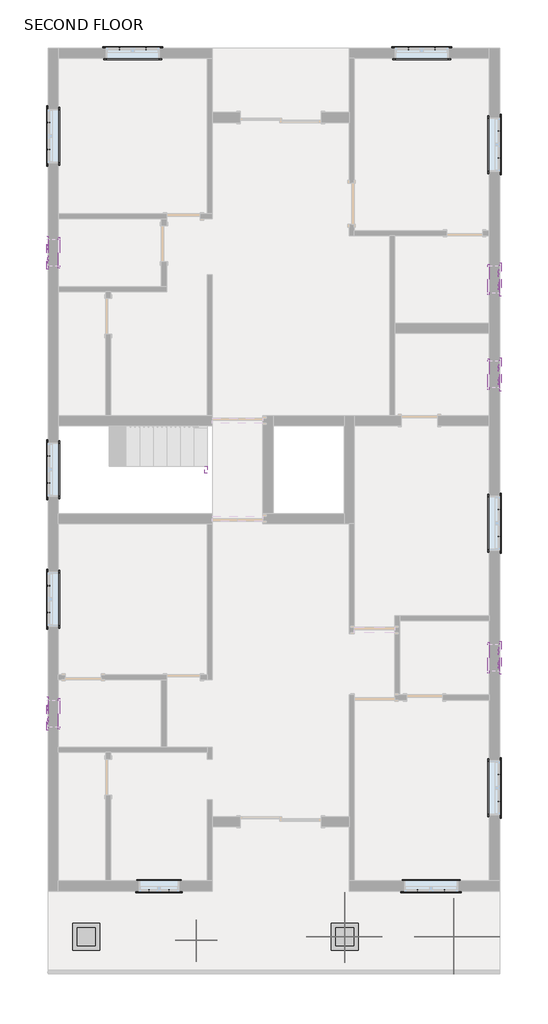
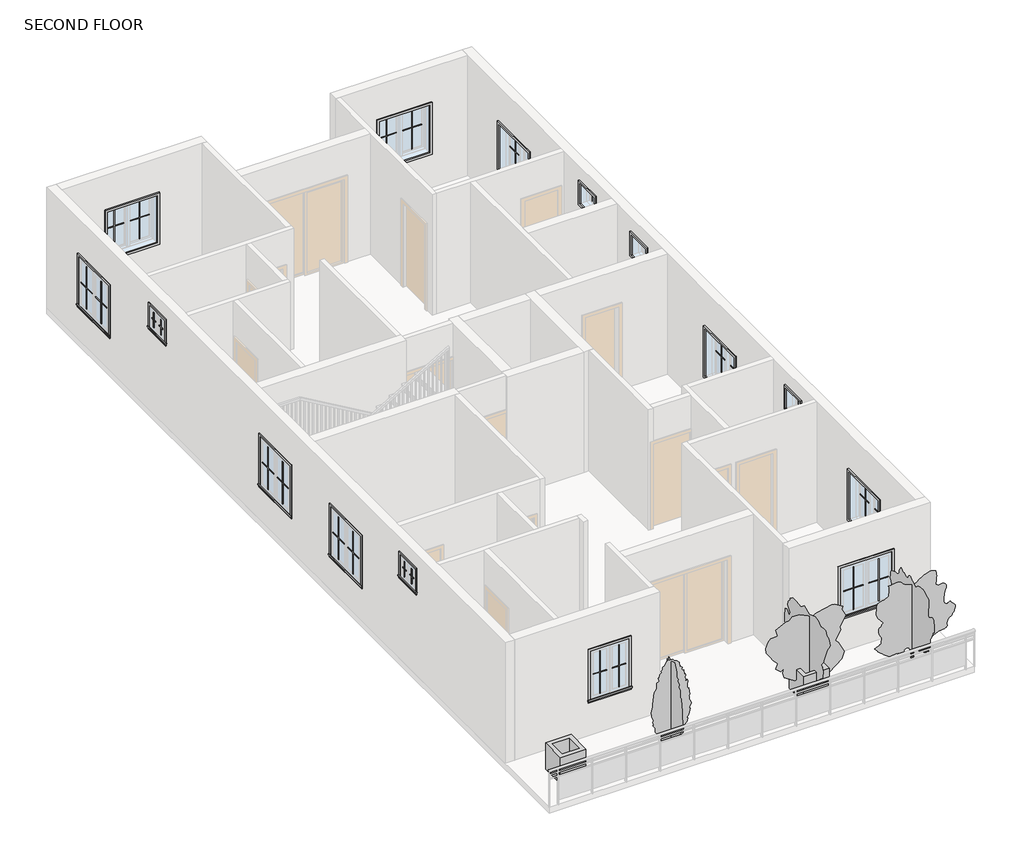
# One storey, part 4 of 4: 60 proxies, 5 geographic elements, 1 railing.
"""IFC4 building model written with IfcOpenShell, lengths in millimetres."""

from ifc_helpers import new_model, si_unit, frame, origin, place, context, project, spatial, polyline, outline, extrude, transform, mapped, element, save
from components import muntin_pattern_2x2_muntin_pattern_2x2_4dfeb3f3, muntin_pattern_2x2_muntin_pattern_2x2_e852a7e4, muntin_pattern_2x2_muntin_pattern_2x2_1acec82f, muntin_pattern_2x2_muntin_pattern_2x2_43d02eee, muntin_pattern_2x2_muntin_pattern_2x2_653c8599, muntin_pattern_2x2_muntin_pattern_2x2_c179cf80, trim_window_exterior_flat_with_sill_7cfdd449, trim_window_exterior_flat_with_sill_e4b28ec3, trim_window_exterior_flat_with_sill_e6f34eb5, trim_window_interior_flat_picture_frame_f1e0b15b, trim_window_interior_flat_picture_frame_39ff4276, trim_window_interior_flat_picture_frame_9a74d23d, planter_2_x2_5b049b04, rpc_tree_conifer_chinese_juniper_7_2_1b9786cd, rpc_tree_fall_american_beech_20_7ed35302, rpc_tree_fall_service_berry_25_c2e4521a

model = new_model("IFC4")

# Units and contexts
model_context = context("Model", 3, world=origin())
ifc_project = project(units=[si_unit("LENGTHUNIT", "METRE", prefix="MILLI")], contexts=[model_context])

# Site, building, storey
site = spatial("IfcSite", under=ifc_project)
building = spatial("IfcBuilding", under=site)
storey = spatial("IfcBuildingStorey", under=building, Name="SECOND FLOOR", Elevation=6400.8)

# Proxies
placement = place(None, origin())
muntin_pattern_2x2_muntin_pattern_2x2_shape = muntin_pattern_2x2_muntin_pattern_2x2_4dfeb3f3(model_context)
element("IfcBuildingElementProxy", 1, Name="Muntin Pattern_2x2 : Muntin Pattern_2x2", ObjectType="Muntin Pattern_2x2 : Muntin Pattern_2x2", at=placement, inside=storey, context=model_context, shape_type="MappedRepresentation", body=[
    mapped(muntin_pattern_2x2_muntin_pattern_2x2_shape, transform((-4756.4414041, 10049.2903263, 7385.05), x_axis=(1.0, 0.0, 0.0), y_axis=(0.0, 1.0, 0.0), z_axis=(0.0, 0.0, 1.0))),
])
element("IfcBuildingElementProxy", 2, Name="Muntin Pattern_2x2 : Muntin Pattern_2x2", ObjectType="Muntin Pattern_2x2 : Muntin Pattern_2x2", at=placement, inside=storey, context=model_context, shape_type="MappedRepresentation", body=[
    mapped(muntin_pattern_2x2_muntin_pattern_2x2_shape, transform((-6348.7039041, 7774.4028263, 7385.05), x_axis=(0.0, 1.0, 0.0), y_axis=(-1.0, 0.0, 0.0), z_axis=(0.0, 0.0, 1.0))),
])
element("IfcBuildingElementProxy", 3, Name="Muntin Pattern_2x2 : Muntin Pattern_2x2", ObjectType="Muntin Pattern_2x2 : Muntin Pattern_2x2", at=placement, inside=storey, context=model_context, shape_type="MappedRepresentation", body=[
    mapped(muntin_pattern_2x2_muntin_pattern_2x2_shape, transform((-6348.7039041, -2664.9971737, 7385.05), x_axis=(0.0, 1.0, 0.0), y_axis=(-1.0, 0.0, 0.0), z_axis=(0.0, 0.0, 1.0))),
])
element("IfcBuildingElementProxy", 4, Name="Muntin Pattern_2x2 : Muntin Pattern_2x2", ObjectType="Muntin Pattern_2x2 : Muntin Pattern_2x2", at=placement, inside=storey, context=model_context, shape_type="MappedRepresentation", body=[
    mapped(muntin_pattern_2x2_muntin_pattern_2x2_shape, transform((2575.0232801, -8930.8596737, 7385.05), x_axis=(-1.0, 0.0, 0.0), y_axis=(0.0, -1.0, 0.0), z_axis=(0.0, 0.0, 1.0))),
])
element("IfcBuildingElementProxy", 5, Name="Muntin Pattern_2x2 : Muntin Pattern_2x2", ObjectType="Muntin Pattern_2x2 : Muntin Pattern_2x2", at=placement, inside=storey, context=model_context, shape_type="MappedRepresentation", body=[
    mapped(muntin_pattern_2x2_muntin_pattern_2x2_shape, transform((3804.9460959, -6313.0721737, 7385.05), x_axis=(0.0, -1.0, 0.0), y_axis=(1.0, 0.0, 0.0), z_axis=(0.0, 0.0, 1.0))),
])
element("IfcBuildingElementProxy", 6, Name="Muntin Pattern_2x2 : Muntin Pattern_2x2", ObjectType="Muntin Pattern_2x2 : Muntin Pattern_2x2", at=placement, inside=storey, context=model_context, shape_type="MappedRepresentation", body=[
    mapped(muntin_pattern_2x2_muntin_pattern_2x2_shape, transform((3804.9460959, -344.0721737, 7385.05), x_axis=(0.0, -1.0, 0.0), y_axis=(1.0, 0.0, 0.0), z_axis=(0.0, 0.0, 1.0))),
])
element("IfcBuildingElementProxy", 7, Name="Muntin Pattern_2x2 : Muntin Pattern_2x2", ObjectType="Muntin Pattern_2x2 : Muntin Pattern_2x2", at=placement, inside=storey, context=model_context, shape_type="MappedRepresentation", body=[
    mapped(muntin_pattern_2x2_muntin_pattern_2x2_shape, transform((3804.9460959, 8190.3278263, 7385.05), x_axis=(0.0, -1.0, 0.0), y_axis=(1.0, 0.0, 0.0), z_axis=(0.0, 0.0, 1.0))),
])
element("IfcBuildingElementProxy", 8, Name="Muntin Pattern_2x2 : Muntin Pattern_2x2", ObjectType="Muntin Pattern_2x2 : Muntin Pattern_2x2", at=placement, inside=storey, context=model_context, shape_type="MappedRepresentation", body=[
    mapped(muntin_pattern_2x2_muntin_pattern_2x2_shape, transform((1758.6585959, 10049.2903263, 7385.05), x_axis=(1.0, 0.0, 0.0), y_axis=(0.0, 1.0, 0.0), z_axis=(0.0, 0.0, 1.0))),
])
element("IfcBuildingElementProxy", 9, Name="Muntin Pattern_2x2 : Muntin Pattern_2x2", ObjectType="Muntin Pattern_2x2 : Muntin Pattern_2x2", at=placement, inside=storey, context=model_context, shape_type="MappedRepresentation", body=[
    mapped(muntin_pattern_2x2_muntin_pattern_2x2_shape, transform((-6348.7039041, 256.0028263, 7385.05), x_axis=(0.0, 1.0, 0.0), y_axis=(-1.0, 0.0, 0.0), z_axis=(0.0, 0.0, 1.0))),
])
muntin_pattern_2x2_muntin_pattern_2x2_2_shape = muntin_pattern_2x2_muntin_pattern_2x2_e852a7e4(model_context)
element("IfcBuildingElementProxy", 10, Name="Muntin Pattern_2x2 : Muntin Pattern_2x2", ObjectType="Muntin Pattern_2x2 : Muntin Pattern_2x2", at=placement, inside=storey, context=model_context, shape_type="MappedRepresentation", body=[
    mapped(muntin_pattern_2x2_muntin_pattern_2x2_2_shape, transform((-4150.0164041, 10049.2903263, 7385.05), x_axis=(-1.0, 0.0, 0.0), y_axis=(0.0, -1.0, 0.0), z_axis=(0.0, 0.0, 1.0))),
])
element("IfcBuildingElementProxy", 11, Name="Muntin Pattern_2x2 : Muntin Pattern_2x2", ObjectType="Muntin Pattern_2x2 : Muntin Pattern_2x2", at=placement, inside=storey, context=model_context, shape_type="MappedRepresentation", body=[
    mapped(muntin_pattern_2x2_muntin_pattern_2x2_2_shape, transform((-6348.7039041, 8380.8278263, 7385.05), x_axis=(0.0, -1.0, 0.0), y_axis=(1.0, 0.0, 0.0), z_axis=(0.0, 0.0, 1.0))),
])
element("IfcBuildingElementProxy", 12, Name="Muntin Pattern_2x2 : Muntin Pattern_2x2", ObjectType="Muntin Pattern_2x2 : Muntin Pattern_2x2", at=placement, inside=storey, context=model_context, shape_type="MappedRepresentation", body=[
    mapped(muntin_pattern_2x2_muntin_pattern_2x2_2_shape, transform((-6348.7039041, -2058.5721737, 7385.05), x_axis=(0.0, -1.0, 0.0), y_axis=(1.0, 0.0, 0.0), z_axis=(0.0, 0.0, 1.0))),
])
element("IfcBuildingElementProxy", 13, Name="Muntin Pattern_2x2 : Muntin Pattern_2x2", ObjectType="Muntin Pattern_2x2 : Muntin Pattern_2x2", at=placement, inside=storey, context=model_context, shape_type="MappedRepresentation", body=[
    mapped(muntin_pattern_2x2_muntin_pattern_2x2_2_shape, transform((1968.5982801, -8930.8596737, 7385.05), x_axis=(1.0, 0.0, 0.0), y_axis=(0.0, 1.0, 0.0), z_axis=(0.0, 0.0, 1.0))),
])
element("IfcBuildingElementProxy", 14, Name="Muntin Pattern_2x2 : Muntin Pattern_2x2", ObjectType="Muntin Pattern_2x2 : Muntin Pattern_2x2", at=placement, inside=storey, context=model_context, shape_type="MappedRepresentation", body=[
    mapped(muntin_pattern_2x2_muntin_pattern_2x2_2_shape, transform((3804.9460959, -6919.4971737, 7385.05), x_axis=(0.0, 1.0, 0.0), y_axis=(-1.0, 0.0, 0.0), z_axis=(0.0, 0.0, 1.0))),
])
element("IfcBuildingElementProxy", 15, Name="Muntin Pattern_2x2 : Muntin Pattern_2x2", ObjectType="Muntin Pattern_2x2 : Muntin Pattern_2x2", at=placement, inside=storey, context=model_context, shape_type="MappedRepresentation", body=[
    mapped(muntin_pattern_2x2_muntin_pattern_2x2_2_shape, transform((3804.9460959, -950.4971737, 7385.05), x_axis=(0.0, 1.0, 0.0), y_axis=(-1.0, 0.0, 0.0), z_axis=(0.0, 0.0, 1.0))),
])
element("IfcBuildingElementProxy", 16, Name="Muntin Pattern_2x2 : Muntin Pattern_2x2", ObjectType="Muntin Pattern_2x2 : Muntin Pattern_2x2", at=placement, inside=storey, context=model_context, shape_type="MappedRepresentation", body=[
    mapped(muntin_pattern_2x2_muntin_pattern_2x2_2_shape, transform((3804.9460959, 7583.9028263, 7385.05), x_axis=(0.0, 1.0, 0.0), y_axis=(-1.0, 0.0, 0.0), z_axis=(0.0, 0.0, 1.0))),
])
element("IfcBuildingElementProxy", 17, Name="Muntin Pattern_2x2 : Muntin Pattern_2x2", ObjectType="Muntin Pattern_2x2 : Muntin Pattern_2x2", at=placement, inside=storey, context=model_context, shape_type="MappedRepresentation", body=[
    mapped(muntin_pattern_2x2_muntin_pattern_2x2_2_shape, transform((2365.0835959, 10049.2903263, 7385.05), x_axis=(-1.0, 0.0, 0.0), y_axis=(0.0, -1.0, 0.0), z_axis=(0.0, 0.0, 1.0))),
])
element("IfcBuildingElementProxy", 18, Name="Muntin Pattern_2x2 : Muntin Pattern_2x2", ObjectType="Muntin Pattern_2x2 : Muntin Pattern_2x2", at=placement, inside=storey, context=model_context, shape_type="MappedRepresentation", body=[
    mapped(muntin_pattern_2x2_muntin_pattern_2x2_2_shape, transform((-6348.7039041, 862.4278263, 7385.05), x_axis=(0.0, -1.0, 0.0), y_axis=(1.0, 0.0, 0.0), z_axis=(0.0, 0.0, 1.0))),
])
muntin_pattern_2x2_muntin_pattern_2x2_3_shape = muntin_pattern_2x2_muntin_pattern_2x2_1acec82f(model_context)
element("IfcBuildingElementProxy", 19, Name="Muntin Pattern_2x2 : Muntin Pattern_2x2", ObjectType="Muntin Pattern_2x2 : Muntin Pattern_2x2", at=placement, inside=storey, context=model_context, shape_type="MappedRepresentation", body=[
    mapped(muntin_pattern_2x2_muntin_pattern_2x2_3_shape, transform((-3635.6664041, -8930.8596737, 7385.05), x_axis=(-1.0, 0.0, 0.0), y_axis=(0.0, -1.0, 0.0), z_axis=(0.0, 0.0, 1.0))),
])
muntin_pattern_2x2_muntin_pattern_2x2_4_shape = muntin_pattern_2x2_muntin_pattern_2x2_43d02eee(model_context)
element("IfcBuildingElementProxy", 20, Name="Muntin Pattern_2x2 : Muntin Pattern_2x2", ObjectType="Muntin Pattern_2x2 : Muntin Pattern_2x2", at=placement, inside=storey, context=model_context, shape_type="MappedRepresentation", body=[
    mapped(muntin_pattern_2x2_muntin_pattern_2x2_4_shape, transform((-4089.6914041, -8930.8596737, 7385.05), x_axis=(1.0, 0.0, 0.0), y_axis=(0.0, 1.0, 0.0), z_axis=(0.0, 0.0, 1.0))),
])
muntin_pattern_2x2_muntin_pattern_2x2_5_shape = muntin_pattern_2x2_muntin_pattern_2x2_653c8599(model_context)
element("IfcBuildingElementProxy", 21, Name="Muntin Pattern_2x2 : Muntin Pattern_2x2", ObjectType="Muntin Pattern_2x2 : Muntin Pattern_2x2", at=placement, inside=storey, context=model_context, shape_type="MappedRepresentation", body=[
    mapped(muntin_pattern_2x2_muntin_pattern_2x2_5_shape, transform((-6348.7039041, 5297.9028263, 8604.25), x_axis=(0.0, 1.0, 0.0), y_axis=(-1.0, 0.0, 0.0), z_axis=(0.0, 0.0, 1.0))),
])
element("IfcBuildingElementProxy", 22, Name="Muntin Pattern_2x2 : Muntin Pattern_2x2", ObjectType="Muntin Pattern_2x2 : Muntin Pattern_2x2", at=placement, inside=storey, context=model_context, shape_type="MappedRepresentation", body=[
    mapped(muntin_pattern_2x2_muntin_pattern_2x2_5_shape, transform((-6348.7039041, -5090.6971737, 8604.25), x_axis=(0.0, 1.0, 0.0), y_axis=(-1.0, 0.0, 0.0), z_axis=(0.0, 0.0, 1.0))),
])
element("IfcBuildingElementProxy", 23, Name="Muntin Pattern_2x2 : Muntin Pattern_2x2", ObjectType="Muntin Pattern_2x2 : Muntin Pattern_2x2", at=placement, inside=storey, context=model_context, shape_type="MappedRepresentation", body=[
    mapped(muntin_pattern_2x2_muntin_pattern_2x2_5_shape, transform((3804.9460959, -3531.7721737, 8604.25), x_axis=(0.0, -1.0, 0.0), y_axis=(1.0, 0.0, 0.0), z_axis=(0.0, 0.0, 1.0))),
])
element("IfcBuildingElementProxy", 24, Name="Muntin Pattern_2x2 : Muntin Pattern_2x2", ObjectType="Muntin Pattern_2x2 : Muntin Pattern_2x2", at=placement, inside=storey, context=model_context, shape_type="MappedRepresentation", body=[
    mapped(muntin_pattern_2x2_muntin_pattern_2x2_5_shape, transform((3804.9460959, 2856.3278263, 8604.25), x_axis=(0.0, -1.0, 0.0), y_axis=(1.0, 0.0, 0.0), z_axis=(0.0, 0.0, 1.0))),
])
element("IfcBuildingElementProxy", 25, Name="Muntin Pattern_2x2 : Muntin Pattern_2x2", ObjectType="Muntin Pattern_2x2 : Muntin Pattern_2x2", at=placement, inside=storey, context=model_context, shape_type="MappedRepresentation", body=[
    mapped(muntin_pattern_2x2_muntin_pattern_2x2_5_shape, transform((3804.9460959, 4996.2778263, 8604.25), x_axis=(0.0, -1.0, 0.0), y_axis=(1.0, 0.0, 0.0), z_axis=(0.0, 0.0, 1.0))),
])
muntin_pattern_2x2_muntin_pattern_2x2_6_shape = muntin_pattern_2x2_muntin_pattern_2x2_c179cf80(model_context)
element("IfcBuildingElementProxy", 26, Name="Muntin Pattern_2x2 : Muntin Pattern_2x2", ObjectType="Muntin Pattern_2x2 : Muntin Pattern_2x2", at=placement, inside=storey, context=model_context, shape_type="MappedRepresentation", body=[
    mapped(muntin_pattern_2x2_muntin_pattern_2x2_6_shape, transform((-6348.7039041, 5599.5278263, 8604.25), x_axis=(0.0, -1.0, 0.0), y_axis=(1.0, 0.0, 0.0), z_axis=(0.0, 0.0, 1.0))),
])
element("IfcBuildingElementProxy", 27, Name="Muntin Pattern_2x2 : Muntin Pattern_2x2", ObjectType="Muntin Pattern_2x2 : Muntin Pattern_2x2", at=placement, inside=storey, context=model_context, shape_type="MappedRepresentation", body=[
    mapped(muntin_pattern_2x2_muntin_pattern_2x2_6_shape, transform((-6348.7039041, -4789.0721737, 8604.25), x_axis=(0.0, -1.0, 0.0), y_axis=(1.0, 0.0, 0.0), z_axis=(0.0, 0.0, 1.0))),
])
element("IfcBuildingElementProxy", 28, Name="Muntin Pattern_2x2 : Muntin Pattern_2x2", ObjectType="Muntin Pattern_2x2 : Muntin Pattern_2x2", at=placement, inside=storey, context=model_context, shape_type="MappedRepresentation", body=[
    mapped(muntin_pattern_2x2_muntin_pattern_2x2_6_shape, transform((3804.9460959, -3833.3971737, 8604.25), x_axis=(0.0, 1.0, 0.0), y_axis=(-1.0, 0.0, 0.0), z_axis=(0.0, 0.0, 1.0))),
])
element("IfcBuildingElementProxy", 29, Name="Muntin Pattern_2x2 : Muntin Pattern_2x2", ObjectType="Muntin Pattern_2x2 : Muntin Pattern_2x2", at=placement, inside=storey, context=model_context, shape_type="MappedRepresentation", body=[
    mapped(muntin_pattern_2x2_muntin_pattern_2x2_6_shape, transform((3804.9460959, 2554.7028263, 8604.25), x_axis=(0.0, 1.0, 0.0), y_axis=(-1.0, 0.0, 0.0), z_axis=(0.0, 0.0, 1.0))),
])
element("IfcBuildingElementProxy", 30, Name="Muntin Pattern_2x2 : Muntin Pattern_2x2", ObjectType="Muntin Pattern_2x2 : Muntin Pattern_2x2", at=placement, inside=storey, context=model_context, shape_type="MappedRepresentation", body=[
    mapped(muntin_pattern_2x2_muntin_pattern_2x2_6_shape, transform((3804.9460959, 4694.6528263, 8604.25), x_axis=(0.0, 1.0, 0.0), y_axis=(-1.0, 0.0, 0.0), z_axis=(0.0, 0.0, 1.0))),
])
trim_window_exterior_flat_with_sill_shape = trim_window_exterior_flat_with_sill_7cfdd449(model_context)
element("IfcBuildingElementProxy", 31, Name="Trim-Window-Exterior-Flat : with Sill", ObjectType="Trim-Window-Exterior-Flat : with Sill", at=placement, inside=storey, context=model_context, shape_type="MappedRepresentation", body=[
    mapped(trim_window_exterior_flat_with_sill_shape, transform((-4453.2289041, 10058.8153263, 8534.4), x_axis=(-1.0, 0.0, 0.0), y_axis=(0.0, 0.0, 1.0), z_axis=(0.0, 1.0, 0.0))),
])
element("IfcBuildingElementProxy", 32, Name="Trim-Window-Exterior-Flat : with Sill", ObjectType="Trim-Window-Exterior-Flat : with Sill", at=placement, inside=storey, context=model_context, shape_type="MappedRepresentation", body=[
    mapped(trim_window_exterior_flat_with_sill_shape, transform((-6358.2289041, 8077.6153263, 8534.4), x_axis=(0.0, -1.0, 0.0), y_axis=(0.0, 0.0, 1.0), z_axis=(-1.0, 0.0, 0.0))),
])
element("IfcBuildingElementProxy", 33, Name="Trim-Window-Exterior-Flat : with Sill", ObjectType="Trim-Window-Exterior-Flat : with Sill", at=placement, inside=storey, context=model_context, shape_type="MappedRepresentation", body=[
    mapped(trim_window_exterior_flat_with_sill_shape, transform((-6358.2289041, -2361.7846737, 8534.4), x_axis=(0.0, -1.0, 0.0), y_axis=(0.0, 0.0, 1.0), z_axis=(-1.0, 0.0, 0.0))),
])
element("IfcBuildingElementProxy", 34, Name="Trim-Window-Exterior-Flat : with Sill", ObjectType="Trim-Window-Exterior-Flat : with Sill", at=placement, inside=storey, context=model_context, shape_type="MappedRepresentation", body=[
    mapped(trim_window_exterior_flat_with_sill_shape, transform((2271.8107801, -8940.3846737, 8534.4), x_axis=(1.0, 0.0, 0.0), y_axis=(0.0, 0.0, 1.0), z_axis=(0.0, -1.0, 0.0))),
])
element("IfcBuildingElementProxy", 35, Name="Trim-Window-Exterior-Flat : with Sill", ObjectType="Trim-Window-Exterior-Flat : with Sill", at=placement, inside=storey, context=model_context, shape_type="MappedRepresentation", body=[
    mapped(trim_window_exterior_flat_with_sill_shape, transform((3814.4710959, -6616.2846737, 8534.4), x_axis=(0.0, 1.0, 0.0), y_axis=(0.0, 0.0, 1.0), z_axis=(1.0, 0.0, 0.0))),
])
element("IfcBuildingElementProxy", 36, Name="Trim-Window-Exterior-Flat : with Sill", ObjectType="Trim-Window-Exterior-Flat : with Sill", at=placement, inside=storey, context=model_context, shape_type="MappedRepresentation", body=[
    mapped(trim_window_exterior_flat_with_sill_shape, transform((3814.4710959, -647.2846737, 8534.4), x_axis=(0.0, 1.0, 0.0), y_axis=(0.0, 0.0, 1.0), z_axis=(1.0, 0.0, 0.0))),
])
element("IfcBuildingElementProxy", 37, Name="Trim-Window-Exterior-Flat : with Sill", ObjectType="Trim-Window-Exterior-Flat : with Sill", at=placement, inside=storey, context=model_context, shape_type="MappedRepresentation", body=[
    mapped(trim_window_exterior_flat_with_sill_shape, transform((3814.4710959, 7887.1153263, 8534.4), x_axis=(0.0, 1.0, 0.0), y_axis=(0.0, 0.0, 1.0), z_axis=(1.0, 0.0, 0.0))),
])
element("IfcBuildingElementProxy", 38, Name="Trim-Window-Exterior-Flat : with Sill", ObjectType="Trim-Window-Exterior-Flat : with Sill", at=placement, inside=storey, context=model_context, shape_type="MappedRepresentation", body=[
    mapped(trim_window_exterior_flat_with_sill_shape, transform((2061.8710959, 10058.8153263, 8534.4), x_axis=(-1.0, 0.0, 0.0), y_axis=(0.0, 0.0, 1.0), z_axis=(0.0, 1.0, 0.0))),
])
element("IfcBuildingElementProxy", 39, Name="Trim-Window-Exterior-Flat : with Sill", ObjectType="Trim-Window-Exterior-Flat : with Sill", at=placement, inside=storey, context=model_context, shape_type="MappedRepresentation", body=[
    mapped(trim_window_exterior_flat_with_sill_shape, transform((-6358.2289041, 559.2153263, 8534.4), x_axis=(0.0, -1.0, 0.0), y_axis=(0.0, 0.0, 1.0), z_axis=(-1.0, 0.0, 0.0))),
])
trim_window_exterior_flat_with_sill_2_shape = trim_window_exterior_flat_with_sill_e4b28ec3(model_context)
element("IfcBuildingElementProxy", 40, Name="Trim-Window-Exterior-Flat : with Sill", ObjectType="Trim-Window-Exterior-Flat : with Sill", at=placement, inside=storey, context=model_context, shape_type="MappedRepresentation", body=[
    mapped(trim_window_exterior_flat_with_sill_2_shape, transform((-3862.6789041, -8940.3846737, 8534.4), x_axis=(1.0, 0.0, 0.0), y_axis=(0.0, 0.0, 1.0), z_axis=(0.0, -1.0, 0.0))),
])
trim_window_exterior_flat_with_sill_3_shape = trim_window_exterior_flat_with_sill_e6f34eb5(model_context)
element("IfcBuildingElementProxy", 41, Name="Trim-Window-Exterior-Flat : with Sill", ObjectType="Trim-Window-Exterior-Flat : with Sill", at=placement, inside=storey, context=model_context, shape_type="MappedRepresentation", body=[
    mapped(trim_window_exterior_flat_with_sill_3_shape, transform((-6358.2289041, 5448.7153263, 9067.8), x_axis=(0.0, -1.0, 0.0), y_axis=(0.0, 0.0, 1.0), z_axis=(-1.0, 0.0, 0.0))),
])
element("IfcBuildingElementProxy", 42, Name="Trim-Window-Exterior-Flat : with Sill", ObjectType="Trim-Window-Exterior-Flat : with Sill", at=placement, inside=storey, context=model_context, shape_type="MappedRepresentation", body=[
    mapped(trim_window_exterior_flat_with_sill_3_shape, transform((-6358.2289041, -4939.8846737, 9067.8), x_axis=(0.0, -1.0, 0.0), y_axis=(0.0, 0.0, 1.0), z_axis=(-1.0, 0.0, 0.0))),
])
element("IfcBuildingElementProxy", 43, Name="Trim-Window-Exterior-Flat : with Sill", ObjectType="Trim-Window-Exterior-Flat : with Sill", at=placement, inside=storey, context=model_context, shape_type="MappedRepresentation", body=[
    mapped(trim_window_exterior_flat_with_sill_3_shape, transform((3814.4710959, -3682.5846737, 9067.8), x_axis=(0.0, 1.0, 0.0), y_axis=(0.0, 0.0, 1.0), z_axis=(1.0, 0.0, 0.0))),
])
element("IfcBuildingElementProxy", 44, Name="Trim-Window-Exterior-Flat : with Sill", ObjectType="Trim-Window-Exterior-Flat : with Sill", at=placement, inside=storey, context=model_context, shape_type="MappedRepresentation", body=[
    mapped(trim_window_exterior_flat_with_sill_3_shape, transform((3814.4710959, 2705.5153263, 9067.8), x_axis=(0.0, 1.0, 0.0), y_axis=(0.0, 0.0, 1.0), z_axis=(1.0, 0.0, 0.0))),
])
element("IfcBuildingElementProxy", 45, Name="Trim-Window-Exterior-Flat : with Sill", ObjectType="Trim-Window-Exterior-Flat : with Sill", at=placement, inside=storey, context=model_context, shape_type="MappedRepresentation", body=[
    mapped(trim_window_exterior_flat_with_sill_3_shape, transform((3814.4710959, 4845.4653263, 9067.8), x_axis=(0.0, 1.0, 0.0), y_axis=(0.0, 0.0, 1.0), z_axis=(1.0, 0.0, 0.0))),
])
trim_window_interior_flat_picture_frame_shape = trim_window_interior_flat_picture_frame_f1e0b15b(model_context)
element("IfcBuildingElementProxy", 46, Name="Trim-Window-Interior-Flat : Picture Frame", ObjectType="Trim-Window-Interior-Flat : Picture Frame", at=placement, inside=storey, context=model_context, shape_type="MappedRepresentation", body=[
    mapped(trim_window_interior_flat_picture_frame_shape, transform((-4453.2289041, 9830.2153263, 8534.4), x_axis=(1.0, 0.0, 0.0), y_axis=(0.0, 0.0, 1.0), z_axis=(0.0, -1.0, 0.0))),
])
element("IfcBuildingElementProxy", 47, Name="Trim-Window-Interior-Flat : Picture Frame", ObjectType="Trim-Window-Interior-Flat : Picture Frame", at=placement, inside=storey, context=model_context, shape_type="MappedRepresentation", body=[
    mapped(trim_window_interior_flat_picture_frame_shape, transform((-6129.6289041, 8077.6153263, 8534.4), x_axis=(0.0, 1.0, 0.0), y_axis=(0.0, 0.0, 1.0), z_axis=(1.0, 0.0, 0.0))),
])
element("IfcBuildingElementProxy", 48, Name="Trim-Window-Interior-Flat : Picture Frame", ObjectType="Trim-Window-Interior-Flat : Picture Frame", at=placement, inside=storey, context=model_context, shape_type="MappedRepresentation", body=[
    mapped(trim_window_interior_flat_picture_frame_shape, transform((-6129.6289041, -2361.7846737, 8534.4), x_axis=(0.0, 1.0, 0.0), y_axis=(0.0, 0.0, 1.0), z_axis=(1.0, 0.0, 0.0))),
])
element("IfcBuildingElementProxy", 49, Name="Trim-Window-Interior-Flat : Picture Frame", ObjectType="Trim-Window-Interior-Flat : Picture Frame", at=placement, inside=storey, context=model_context, shape_type="MappedRepresentation", body=[
    mapped(trim_window_interior_flat_picture_frame_shape, transform((2271.8107801, -8711.7846737, 8534.4), x_axis=(-1.0, 0.0, 0.0), y_axis=(0.0, 0.0, 1.0), z_axis=(0.0, 1.0, 0.0))),
])
element("IfcBuildingElementProxy", 50, Name="Trim-Window-Interior-Flat : Picture Frame", ObjectType="Trim-Window-Interior-Flat : Picture Frame", at=placement, inside=storey, context=model_context, shape_type="MappedRepresentation", body=[
    mapped(trim_window_interior_flat_picture_frame_shape, transform((3585.8710959, -6616.2846737, 8534.4), x_axis=(0.0, -1.0, 0.0), y_axis=(0.0, 0.0, 1.0), z_axis=(-1.0, 0.0, 0.0))),
])
element("IfcBuildingElementProxy", 51, Name="Trim-Window-Interior-Flat : Picture Frame", ObjectType="Trim-Window-Interior-Flat : Picture Frame", at=placement, inside=storey, context=model_context, shape_type="MappedRepresentation", body=[
    mapped(trim_window_interior_flat_picture_frame_shape, transform((3585.8710959, -647.2846737, 8534.4), x_axis=(0.0, -1.0, 0.0), y_axis=(0.0, 0.0, 1.0), z_axis=(-1.0, 0.0, 0.0))),
])
element("IfcBuildingElementProxy", 52, Name="Trim-Window-Interior-Flat : Picture Frame", ObjectType="Trim-Window-Interior-Flat : Picture Frame", at=placement, inside=storey, context=model_context, shape_type="MappedRepresentation", body=[
    mapped(trim_window_interior_flat_picture_frame_shape, transform((3585.8710959, 7887.1153263, 8534.4), x_axis=(0.0, -1.0, 0.0), y_axis=(0.0, 0.0, 1.0), z_axis=(-1.0, 0.0, 0.0))),
])
element("IfcBuildingElementProxy", 53, Name="Trim-Window-Interior-Flat : Picture Frame", ObjectType="Trim-Window-Interior-Flat : Picture Frame", at=placement, inside=storey, context=model_context, shape_type="MappedRepresentation", body=[
    mapped(trim_window_interior_flat_picture_frame_shape, transform((2061.8710959, 9830.2153263, 8534.4), x_axis=(1.0, 0.0, 0.0), y_axis=(0.0, 0.0, 1.0), z_axis=(0.0, -1.0, 0.0))),
])
element("IfcBuildingElementProxy", 54, Name="Trim-Window-Interior-Flat : Picture Frame", ObjectType="Trim-Window-Interior-Flat : Picture Frame", at=placement, inside=storey, context=model_context, shape_type="MappedRepresentation", body=[
    mapped(trim_window_interior_flat_picture_frame_shape, transform((-6129.6289041, 559.2153263, 8534.4), x_axis=(0.0, 1.0, 0.0), y_axis=(0.0, 0.0, 1.0), z_axis=(1.0, 0.0, 0.0))),
])
trim_window_interior_flat_picture_frame_2_shape = trim_window_interior_flat_picture_frame_39ff4276(model_context)
element("IfcBuildingElementProxy", 55, Name="Trim-Window-Interior-Flat : Picture Frame", ObjectType="Trim-Window-Interior-Flat : Picture Frame", at=placement, inside=storey, context=model_context, shape_type="MappedRepresentation", body=[
    mapped(trim_window_interior_flat_picture_frame_2_shape, transform((-3862.6789041, -8711.7846737, 8534.4), x_axis=(-1.0, 0.0, 0.0), y_axis=(0.0, 0.0, 1.0), z_axis=(0.0, 1.0, 0.0))),
])
trim_window_interior_flat_picture_frame_3_shape = trim_window_interior_flat_picture_frame_9a74d23d(model_context)
element("IfcBuildingElementProxy", 56, Name="Trim-Window-Interior-Flat : Picture Frame", ObjectType="Trim-Window-Interior-Flat : Picture Frame", at=placement, inside=storey, context=model_context, shape_type="MappedRepresentation", body=[
    mapped(trim_window_interior_flat_picture_frame_3_shape, transform((-6129.6289041, 5448.7153263, 9067.8), x_axis=(0.0, 1.0, 0.0), y_axis=(0.0, 0.0, 1.0), z_axis=(1.0, 0.0, 0.0))),
])
element("IfcBuildingElementProxy", 57, Name="Trim-Window-Interior-Flat : Picture Frame", ObjectType="Trim-Window-Interior-Flat : Picture Frame", at=placement, inside=storey, context=model_context, shape_type="MappedRepresentation", body=[
    mapped(trim_window_interior_flat_picture_frame_3_shape, transform((-6129.6289041, -4939.8846737, 9067.8), x_axis=(0.0, 1.0, 0.0), y_axis=(0.0, 0.0, 1.0), z_axis=(1.0, 0.0, 0.0))),
])
element("IfcBuildingElementProxy", 58, Name="Trim-Window-Interior-Flat : Picture Frame", ObjectType="Trim-Window-Interior-Flat : Picture Frame", at=placement, inside=storey, context=model_context, shape_type="MappedRepresentation", body=[
    mapped(trim_window_interior_flat_picture_frame_3_shape, transform((3585.8710959, -3682.5846737, 9067.8), x_axis=(0.0, -1.0, 0.0), y_axis=(0.0, 0.0, 1.0), z_axis=(-1.0, 0.0, 0.0))),
])
element("IfcBuildingElementProxy", 59, Name="Trim-Window-Interior-Flat : Picture Frame", ObjectType="Trim-Window-Interior-Flat : Picture Frame", at=placement, inside=storey, context=model_context, shape_type="MappedRepresentation", body=[
    mapped(trim_window_interior_flat_picture_frame_3_shape, transform((3585.8710959, 2705.5153263, 9067.8), x_axis=(0.0, -1.0, 0.0), y_axis=(0.0, 0.0, 1.0), z_axis=(-1.0, 0.0, 0.0))),
])
element("IfcBuildingElementProxy", 60, Name="Trim-Window-Interior-Flat : Picture Frame", ObjectType="Trim-Window-Interior-Flat : Picture Frame", at=placement, inside=storey, context=model_context, shape_type="MappedRepresentation", body=[
    mapped(trim_window_interior_flat_picture_frame_3_shape, transform((3585.8710959, 4845.4653263, 9067.8), x_axis=(0.0, -1.0, 0.0), y_axis=(0.0, 0.0, 1.0), z_axis=(-1.0, 0.0, 0.0))),
])

# Geographic elements
planter_2_x2_shape = planter_2_x2_5b049b04(model_context)
element("IfcGeographicElement", 61, ObjectType="Planter : 2'X2'", at=placement, inside=storey, context=model_context, shape_type="MappedRepresentation", body=[
    mapped(planter_2_x2_shape, transform((-5500.9789041, -9969.0846737, 6400.8), x_axis=(1.0, 0.0, 0.0), y_axis=(0.0, 1.0, 0.0), z_axis=(0.0, 0.0, 1.0))),
])
element("IfcGeographicElement", 62, ObjectType="Planter : 2'X2'", at=placement, inside=storey, context=model_context, shape_type="MappedRepresentation", body=[
    mapped(planter_2_x2_shape, transform((328.3210959, -9969.0846737, 6400.8), x_axis=(1.0, 0.0, 0.0), y_axis=(0.0, 1.0, 0.0), z_axis=(0.0, 0.0, 1.0))),
])
rpc_tree_conifer_chinese_juniper_7_2_shape = rpc_tree_conifer_chinese_juniper_7_2_1b9786cd(model_context)
element("IfcGeographicElement", 63, ObjectType="RPC Tree - Conifer : Chinese Juniper - 7' 2", at=placement, inside=storey, context=model_context, shape_type="MappedRepresentation", body=[
    mapped(rpc_tree_conifer_chinese_juniper_7_2_shape, transform((-3024.6755752, -10045.2846737, 6400.8), x_axis=(1.0, 0.0, 0.0), y_axis=(0.0, 1.0, 0.0), z_axis=(0.0, 0.0, 1.0))),
])
rpc_tree_fall_american_beech_20_shape = rpc_tree_fall_american_beech_20_7ed35302(model_context)
element("IfcGeographicElement", 64, ObjectType="RPC Tree - Fall : American Beech - 20'", at=placement, inside=storey, context=model_context, shape_type="MappedRepresentation", body=[
    mapped(rpc_tree_fall_american_beech_20_shape, transform((2785.7710959, -9969.0846737, 6400.8), x_axis=(1.0, 0.0, 0.0), y_axis=(0.0, 1.0, 0.0), z_axis=(0.0, 0.0, 1.0))),
])
rpc_tree_fall_service_berry_25_shape = rpc_tree_fall_service_berry_25_c2e4521a(model_context)
element("IfcGeographicElement", 65, ObjectType="RPC Tree - Fall : Service Berry - 25'", at=placement, inside=storey, context=model_context, shape_type="MappedRepresentation", body=[
    mapped(rpc_tree_fall_service_berry_25_shape, transform((328.3210959, -9969.0846737, 6400.8), x_axis=(1.0, 0.0, 0.0), y_axis=(0.0, 1.0, 0.0), z_axis=(0.0, 0.0, 1.0))),
])

# Railing
element("IfcRailing", 66, ObjectType="Handrail - Rectangular", at=placement, inside=storey, context=model_context, shape_type="SweptSolid", body=[
    extrude(outline(polyline([(-2827.6289041, 635.4153263), (-2776.8289041, 635.4153263), (-2776.8289041, 483.0153263), (-2827.6289041, 483.0153263), (-2827.6289041, 635.4153263)])), frame((0.0, 0.0, 8864.6), z_axis=(0.0, 0.0, 1.0), x_axis=(1.0, 0.0, 0.0)), (0.0, 0.0, 1.0), 50.8),
    extrude(outline(polyline([(-2792.7039041, 543.3403263), (-2792.7039041, 524.2903263), (-2811.7539041, 524.2903263), (-2811.7539041, 543.3403263), (-2792.7039041, 543.3403263)])), frame((0.0, 0.0, 8001.0), z_axis=(0.0, 0.0, 1.0), x_axis=(1.0, 0.0, 0.0)), (0.0, 0.0, 1.0), 863.6),
    extrude(outline(polyline([(-2792.7039041, 502.0653263), (-2792.7039041, 483.0153263), (-2811.7539041, 483.0153263), (-2811.7539041, 502.0653263), (-2792.7039041, 502.0653263)])), frame((0.0, 0.0, 8001.0), z_axis=(0.0, 0.0, 1.0), x_axis=(1.0, 0.0, 0.0)), (0.0, 0.0, 1.0), 863.6),
    extrude(outline(polyline([(-2792.7039041, 635.4153263), (-2792.7039041, 616.3653263), (-2811.7539041, 616.3653263), (-2811.7539041, 635.4153263), (-2792.7039041, 635.4153263)])), frame((0.0, 0.0, 8001.0), z_axis=(0.0, 0.0, 1.0), x_axis=(1.0, 0.0, 0.0)), (0.0, 0.0, 1.0), 863.6),
])

save(model, "model.ifc")

# Revit data of these elements
# Type "Muntin Pattern_2x2 : Muntin Pattern_2x2"
#   Width [instance default] = 4' - 0"
#   Thickness = 0' - 0 1/2"
#   Height [instance default] = 4' - 0"
#   Distance = 0' - 0 3/4"
#   Interior Material [instance default] = none
#   Exterior Material [instance default] = none
#   Default Elevation = 0
# Type "Trim-Window-Exterior-Flat : with Sill"
#   Trim Width = 0' - 2 1/4"
#   Trim Thickness_Picture Frame = 0' - 1 1/4"
#   Trim Thickness_with Sill = 0' - 0 3/4"
#   Sill Thickness = 0' - 1 1/4"
#   Opening Width [instance default] = 2' - 0"
#   Opening Height [instance default] = 3' - 0"
#   Default Elevation = 4' - 0"
#   Sill = yes
#   Picture Frame = no
#   Trim Material [instance default] = none
# Type "Trim-Window-Interior-Flat : Picture Frame"
#   Trim Thickness_Picture Frame = 0' - 1 1/4"
#   Trim Width = 0' - 2 1/4"
#   Trim Thickness_with Sill = 0' - 0 3/4"
#   Sill Thickness = 0' - 1 1/4"
#   Opening Width [instance default] = 2' - 0"
#   Opening Height [instance default] = 3' - 0"
#   Default Elevation = 4' - 0"
#   Sill = no
#   Picture Frame = yes
#   Trim Material [instance default] = none
# Type "Planter : 2'X2'"
#   Depth = 2' - 0"
#   Height = 2' - 6"
#   Width = 2' - 0"
#   Material = Concrete, Precast
# Type "RPC Tree - Conifer : Chinese Juniper - 7' 2"
#   built-in parameter 1005198 = "{2, 15},{39, RPC-16-FUM3-UUQ0-UBF0-N000-ST1L-LVER-AU},{1, 0},{1, 0},{2, 35},{1, 8},{5, Color},{1, 0},{1, 0},{3, 0.8},{3, 0.8},{3, 0.8},{1, 8},{7, BBoxMin},{1, 0},{1, 0},{1, 0},{1, 0},{1, 0},{1, 8},{7, BBoxMax},{1, 0},{1, 0},{1, 0},{1, 0},{1, 0},{2, 11},{9, RPCTypeId},{1, 0},{1, 0},{39, RPC-16-FUM3-UUQ0-UBF0-N000-ST1L-LVER-AU},{1, 6},{14, RPCPlantHeight},{1, 0},{1, 0},{1, 7},{2, 11},{7, keyword},{1, 0},{1, 0},{96, :Geometry:RPC:Chinese Juniper:juniperus chinensis:chinese:juniper:cupressaceae:conifer:evergreen},{2, 11},{8, category},{1, 0},{1, 0},{16, :Trees [General]},{2, 11},{12, LocalizedUID},{1, 0},{1, 0},{15, Chinese Juniper},{2, 14},{6, Height},{1, 0},{1, 0},{1, 7},{1, 2},{16, Cast Reflections},{1, 0},{1, 0},{1, 0},{1, 2},{12, Cast Shadows},{1, 0},{1, 0},{1, 1},{1, 2},{9, Lock View},{1, 0},{1, 0},{1, 0},{1, 4},{5, ViewC},{1, 0},{1, 0},{1, 0},{2, 11},{20, AdvancedUIDefinition},{1, 0},{1, 0},{0, },{2, 11},{10, AssetLibID},{1, 0},{1, 0},{36, 4D3F6E72-3F99-4203-98E9-AF80B3C7A7A4},{2, 11},{10, BaseSchema},{1, 0},{1, 0},{9, RPCSchema},{2, 11},{12, ExchangeGUID},{1, 0},{1, 0},{0, },{1, 2},{6, Hidden},{1, 0},{1, 0},{1, 0},{1, 4},{11, RPCCategory},{1, 0},{1, 0},{1, 0},{2, 11},{8, RPCImage},{1, 0},{1, 0},{0, },{1, 4},{13, SchemaVersion},{1, 0},{1, 0},{1, 4},{2, 11},{12, UIDefinition},{1, 0},{1, 0},{0, },{2, 11},{6, UIName},{1, 0},{1, 0},{39, RPC-16-FUM3-UUQ0-UBF0-N000-ST1L-LVER-AU},{2, 11},{11, VersionGUID},{1, 0},{1, 0},{9, RPCSchema},{2, 11},{9, assettype},{1, 0},{1, 0},{11, RPCGeometry},{2, 11},{11, description},{1, 0},{1, 0},{0, },{2, 11},{9, localname},{1, 0},{1, 0},{3, RPC},{2, 11},{9, localtype},{1, 0},{1, 0},{3, RPC},{1, 4},{8, revision},{1, 0},{1, 0},{1, 1},{2, 11},{9, thumbnail},{1, 0},{1, 0},{0, },{1, 4},{7, version},{1, 0},{1, 0},{1, 1},{1, 2},{20, RPC_Cast Reflections},{1, 0},{1, 0},{1, 1},{1, 2},{16, RPC_Cast Shadows},{1, 0},{1, 0},{1, 1},{1, 2},{13, RPC_Lock View},{1, 0},{1, 0},{1, 0},{1, 4},{9, RPC_ViewC},{1, 0},{1, 0},{1, 0},{21, assetlibrary_base.fbx},{1, 5},"
#   built-in parameter 1005195 = "RPC-16-FUM3-UUQ0-UBF0-N000-ST1L-LVER-AU"
#   Type Comments = "Chinese Juniper"
#   Assembly Code = "G2050500"
#   Height = 7' - 0"
#   Description = (empty or 0)
#   Default Elevation = 0
# Type "RPC Tree - Fall : American Beech - 20'"
#   built-in parameter 1005198 = "{2, 15},{39, RPC-16-G2VX-NFFX-5QM5-6000-ST1L-LVER-AU},{1, 0},{1, 0},{2, 13},{1, 8},{5, Color},{1, 0},{1, 0},{3, 0.8},{3, 0.8},{3, 0.8},{1, 8},{7, BBoxMin},{1, 0},{1, 0},{1, 0},{1, 0},{1, 0},{1, 8},{7, BBoxMax},{1, 0},{1, 0},{1, 0},{1, 0},{1, 0},{2, 11},{9, RPCTypeId},{1, 0},{1, 0},{39, RPC-16-G2VX-NFFX-5QM5-6000-ST1L-LVER-AU},{1, 6},{14, RPCPlantHeight},{1, 0},{1, 0},{2, 20},{2, 11},{7, keyword},{1, 0},{1, 0},{39, :RPCs:Fall Trees [General]:Geometry:RPC},{2, 11},{8, category},{1, 0},{1, 0},{20, Fall Trees [General]},{2, 11},{12, LocalizedUID},{1, 0},{1, 0},{21, American Beech [Fall]},{2, 14},{6, Height},{1, 0},{1, 0},{2, 20},{1, 2},{16, Cast Reflections},{1, 0},{1, 0},{1, 0},{1, 2},{12, Cast Shadows},{1, 0},{1, 0},{1, 1},{1, 2},{9, Lock View},{1, 0},{1, 0},{1, 0},{1, 4},{5, ViewC},{1, 0},{1, 0},{1, 0},{21, assetlibrary_base.fbx},{1, 5},"
#   built-in parameter 1005195 = "RPC-16-G2VX-NFFX-5QM5-6000-ST1L-LVER-AU"
#   Type Comments = "American Beech"
#   Assembly Code = "G2050500"
#   Height = 7' - 0"
#   Default Elevation = 0
# Type "RPC Tree - Fall : Service Berry - 25'"
#   built-in parameter 1005198 = "{2, 15},{39, RPC-16-FVGU-8VG0-7PL0-4000-ST1L-LVER-AU},{1, 0},{1, 0},{2, 13},{1, 8},{5, Color},{1, 0},{1, 0},{3, 0.8},{3, 0.8},{3, 0.8},{1, 8},{7, BBoxMin},{1, 0},{1, 0},{1, 0},{1, 0},{1, 0},{1, 8},{7, BBoxMax},{1, 0},{1, 0},{1, 0},{1, 0},{1, 0},{2, 11},{9, RPCTypeId},{1, 0},{1, 0},{39, RPC-16-FVGU-8VG0-7PL0-4000-ST1L-LVER-AU},{1, 6},{14, RPCPlantHeight},{1, 0},{1, 0},{2, 25},{2, 11},{7, keyword},{1, 0},{1, 0},{39, :RPCs:Fall Trees [General]:Geometry:RPC},{2, 11},{8, category},{1, 0},{1, 0},{20, Fall Trees [General]},{2, 11},{12, LocalizedUID},{1, 0},{1, 0},{20, Service Berry [Fall]},{2, 14},{6, Height},{1, 0},{1, 0},{2, 25},{1, 2},{16, Cast Reflections},{1, 0},{1, 0},{1, 0},{1, 2},{12, Cast Shadows},{1, 0},{1, 0},{1, 1},{1, 2},{9, Lock View},{1, 0},{1, 0},{1, 0},{1, 4},{5, ViewC},{1, 0},{1, 0},{1, 0},{21, assetlibrary_base.fbx},{1, 5},"
#   built-in parameter 1005195 = "RPC-16-FVGU-8VG0-7PL0-4000-ST1L-LVER-AU"
#   Type Comments = "Service Berry"
#   Assembly Code = "G2050500"
#   Height = 7' - 0"
#   Default Elevation = 0
# Type "Handrail - Rectangular"
#   Assembly Code = "C2010400"
#   built-in parameter 1008612 = 0.0416667 (stored number, unit not read)
#   built-in parameter 1008611 = 0.0416667 (stored number, unit not read)
#   built-in parameter 1008609 = 0.333333 (stored number, unit not read)
#   built-in parameter 1008604 = 0.166667 (stored number, unit not read)
#   built-in parameter 1008603 = 0.166667 (stored number, unit not read)
#   Railing Height = 3' - 0"
#   built-in parameter 1008630 = 2
#   built-in parameter 1008610 = 2
#   built-in parameter 1008618 = Baluster - Square : 3/4"
# Elements 1, 2, 3, 4, 5, 6, 7, 8, 9, 10, 11, 12, 13, 14, 15, 16, 17, 18 (IfcBuildingElementProxy, "Muntin Pattern_2x2 : Muntin Pattern_2x2")
#   Width = 1' - 6 5/8"
#   Height = 3' - 6 1/2"
#   Interior Material = Wood - Stained
#   Exterior Material = Clad - White
#   Phase Created = New Construction
#   Materials on its faces: "Clad - White", "Wood - Stained"
# Elements 19, 20 (IfcBuildingElementProxy, "Muntin Pattern_2x2 : Muntin Pattern_2x2")
#   Width = 1' - 0 5/8"
#   Height = 3' - 6 1/2"
#   Interior Material = Wood - Stained
#   Exterior Material = Clad - White
#   Phase Created = New Construction
#   Materials on its faces: "Clad - White", "Wood - Stained"
# Elements 21, 22, 23, 24, 25, 26, 27, 28, 29, 30 (IfcBuildingElementProxy, "Muntin Pattern_2x2 : Muntin Pattern_2x2")
#   Width = 0' - 6 5/8"
#   Height = 1' - 3 1/2"
#   Interior Material = Wood - Stained
#   Exterior Material = Clad - White
#   Phase Created = New Construction
#   Materials on its faces: "Clad - White", "Wood - Stained"
# Elements 31, 32, 33, 34, 35, 36, 37, 38, 39 (IfcBuildingElementProxy, "Trim-Window-Exterior-Flat : with Sill")
#   Opening Width = 4' - 0"
#   Opening Height = 4' - 0"
#   Trim Material = Clad - White
#   Phase Created = New Construction
#   Materials on its faces: "Clad - White"
# Element 40 (IfcBuildingElementProxy, "Trim-Window-Exterior-Flat : with Sill")
#   Opening Width = 3' - 0"
#   Opening Height = 4' - 0"
#   Trim Material = Clad - White
#   Phase Created = New Construction
#   Materials on its faces: "Clad - White"
# Elements 41, 42, 43, 44, 45 (IfcBuildingElementProxy, "Trim-Window-Exterior-Flat : with Sill")
#   Opening Width = 2' - 0"
#   Opening Height = 1' - 9"
#   Trim Material = Clad - White
#   Phase Created = New Construction
#   Materials on its faces: "Clad - White"
# Elements 46, 47, 48, 49, 50, 51, 52, 53, 54 (IfcBuildingElementProxy, "Trim-Window-Interior-Flat : Picture Frame")
#   Opening Width = 4' - 0"
#   Opening Height = 4' - 0"
#   Trim Material = Wood - Stained
#   Phase Created = New Construction
#   Materials on its faces: "Wood - Stained"
# Element 55 (IfcBuildingElementProxy, "Trim-Window-Interior-Flat : Picture Frame")
#   Opening Width = 3' - 0"
#   Opening Height = 4' - 0"
#   Trim Material = Wood - Stained
#   Phase Created = New Construction
#   Materials on its faces: "Wood - Stained"
# Elements 56, 57, 58, 59, 60 (IfcBuildingElementProxy, "Trim-Window-Interior-Flat : Picture Frame")
#   Opening Width = 2' - 0"
#   Opening Height = 1' - 9"
#   Trim Material = Wood - Stained
#   Phase Created = New Construction
#   Materials on its faces: "Wood - Stained"
# Elements 61, 62 (IfcGeographicElement, "Planter : 2'X2'")
#   Phase Created = New Construction
#   Materials on its faces: "Concrete, Precast"
# Element 63 (IfcGeographicElement, "RPC Tree - Conifer : Chinese Juniper - 7' 2")
#   Phase Created = New Construction
# Element 64 (IfcGeographicElement, "RPC Tree - Fall : American Beech - 20'")
#   Phase Created = New Construction
# Element 65 (IfcGeographicElement, "RPC Tree - Fall : Service Berry - 25'")
#   Phase Created = New Construction
# Element 66 (IfcRailing, "Handrail - Rectangular")
#   Phase Created = New Construction
# Materials
#   "Concrete, Precast": class "Concrete", colour RGB 198 187 187, transparency 0, Description = "Precast concrete", Cost = 0
#   "Clad - White": class "Wood", colour RGB 242 242 238, transparency 0, Cost = 0
#   "Wood - Stained": class "Wood", colour RGB 224 178 126, transparency 0, Cost = 0
